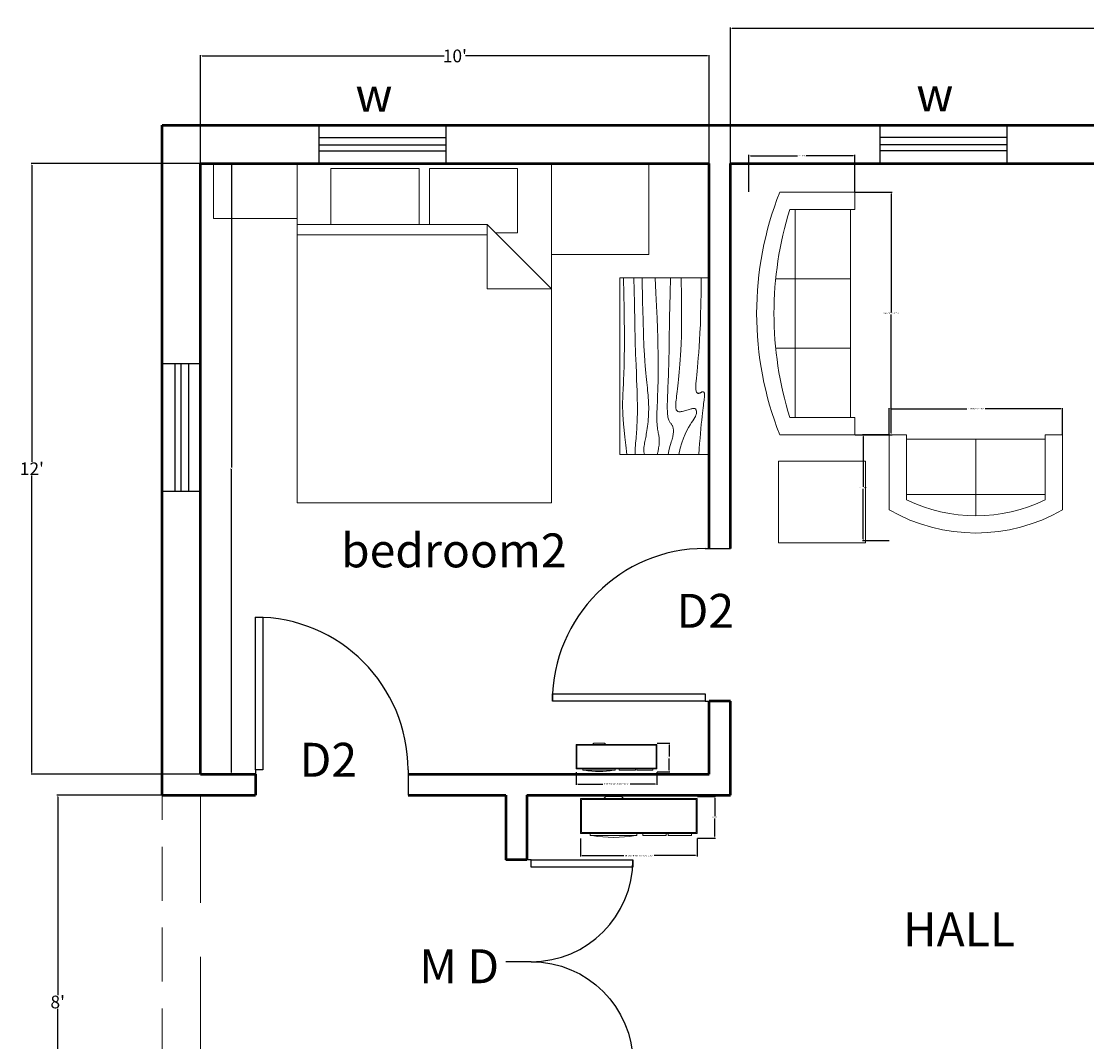
# Model space of a CAD drawing. Units: inches. Extents: x -10 to 557, y -66 to 886.
# Tile 2 of 6: x -10 to 241, y 207 to 448. Entities that reach past the tile are written whole.
import ezdxf

# ---------------------------------------------------------------- set-up
doc = ezdxf.new("R2010")
doc.units = ezdxf.units.IN
doc.header["$MEASUREMENT"] = 0
doc.linetypes.add('DASHED', pattern=[19.05, 12.7, -6.35])
for name, color, linetype, lineweight in [('A-ANNO-DIMS', 2, 'Continuous', 18), ('A-ANNO-TEXT', 7, 'Continuous', 18), ('A-AREA-IDEN', 7, 'Continuous', 25), ('A-DOOR', 4, 'Continuous', 25), ('A-FURN', 8, 'Continuous', 18), ('A-GLAZ', 4, 'Continuous', 25), ('A-WALL', 7, 'Continuous', 50), ('A-WALL-OVHD', 8, 'DASHED', 18)]:
    doc.layers.add(name, color=color, linetype=linetype, lineweight=lineweight)
doc.styles.get("Standard").update_dxf_attribs({"font": 'arial.ttf'})
doc.dimstyles.get("Standard").update_dxf_attribs({"dimtxt": 0.3, "dimasz": 0.4, "dimexe": 0.18, "dimexo": 0.0625, "dimgap": 0.09, "dimtad": 0, "dimtih": 1, "dimtoh": 1, "dimdec": 0, "dimrnd": 8, "dimzin": 0, "dimdsep": 46, "dimlunit": 3, "dimtxsty": 'Standard', "dimcen": 0.09, "dimadec": 0, "dimazin": 0, "dimtfac": 1, "dimtdec": 0, "dimtofl": 0, "dimtmove": 0, "dimatfit": 3, "dimfxl": 1, "dimtolj": 1, "dimtzin": 0, "dimarcsym": 0})

# ---------------------------------------------------------------- blocks, each defined once
blk = doc.blocks.new('*U32')
for p, q in [((0, 0), (0, -6)), ((36, 0), (36, -6))]:
    blk.add_line(p, q)
blk.add_lwpolyline([(0, 0), (0, 36), (1.75, 36), (1.75, 0)], close=True)
blk.add_arc((0, 0), 36, 0, 90)
blk = doc.blocks.new('*U33')
for p, q in [((0, 0), (0, -6)), ((24, 0), (24, -6))]:
    blk.add_line(p, q)
blk.add_lwpolyline([(0, 0), (0, 24), (1.75, 24), (1.75, 0)], close=True)
blk.add_arc((0, 0), 24, 0, 90)
blk = doc.blocks.new('Bed - Queen')
for p, q in [((0, -80.00003), (0, 0)), ((0, 0), (59.99999, 0)), ((59.99999, 0), (59.99999, -80.00003)), ((7.99999, -1.2), (28.79998, -1.2)), ((7.99999, -14.4), (7.99999, -1.2)), ((28.79998, -1.2), (28.79998, -14.4)), ((31.19999, -1.2), (51.99999, -1.2)), ((31.19999, -14.4), (31.19999, -1.2)), ((51.99999, -1.2), (51.99999, -16.4)), ((0, -14.4), (44.8, -14.4)), ((59.99999, -29.6), (44.8, -14.4)), ((44.8, -14.4), (44.8, -29.6)), ((44.8, -16.8), (0, -16.8)), ((51.99999, -16.4), (46.79936, -16.4)), ((44.8, -29.6), (59.99999, -29.6)), ((59.99999, -80.00003), (0, -80.00003))]:
    blk.add_line(p, q)
blk = doc.blocks.new('Table - Rectangular Woodgrain 60 x 30 in.')
for p, q in [((0, 0), (0, -30)), ((60, 0), (0, 0)), ((60, -30), (60, 0)), ((0, -30), (60, -30))]:
    blk.add_line(p, q)
for points in [[(0, -2.4), (4.8155, -2.418), (9.0302, -2.4688), (12.709, -2.5477), (15.9167, -2.65), (18.7181, -2.7711), (21.1781, -2.9063), (23.3616, -3.0508), (25.3333, -3.2), (27.1477, -3.3495), (28.8172, -3.4958), (30.3437, -3.636), (31.7291, -3.7667), (32.9756, -3.8849), (34.0849, -3.9875), (35.059, -4.0714), (35.9, -4.1334), (36.6114, -4.1711), (37.2041, -4.1854), (37.6906, -4.1779), (38.0833, -4.15), (38.3948, -4.1034), (38.6375, -4.0396), (38.8239, -3.9602), (38.9666, -3.8667), (39.0764, -3.7608), (39.1573, -3.6448), (39.2116, -3.521), (39.2416, -3.3917), (39.2498, -3.2593), (39.2385, -3.1261), (39.21, -2.9944), (39.1666, -2.8667), (39.111, -2.7447), (39.0468, -2.6281), (38.978, -2.5163), (38.9083, -2.4083), (38.8418, -2.3035), (38.7823, -2.201), (38.7337, -2.1001), (38.7, -2), (38.6844, -1.9003), (38.6875, -1.8021), (38.7094, -1.707), (38.75, -1.6167), (38.8094, -1.5326), (38.8875, -1.4563), (38.9844, -1.3893), (39.1, -1.3333), (39.2351, -1.2896), (39.3937, -1.2583), (39.5804, -1.2396), (39.8, -1.2333), (40.057, -1.2396), (40.3562, -1.2583), (40.7023, -1.2896), (41.1, -1.3333), (41.5547, -1.3895), (42.0755, -1.4573), (42.6721, -1.5361), (43.3542, -1.625), (44.1316, -1.7233), (45.014, -1.8302), (46.0114, -1.9449), (47.1333, -2.0667), (48.3862, -2.1947), (49.7625, -2.3281), (51.2513, -2.4663), (52.8416, -2.6083), (54.5226, -2.7535), (56.2833, -2.9011), (58.1127, -3.0501), (60, -3.2)], [(0, -9.2), (6.5759, -9.0858), (11.9385, -9.0365), (16.2527, -9.0418), (19.6833, -9.0917), (22.3952, -9.1759), (24.5531, -9.2844), (26.322, -9.4069), (27.8666, -9.5333), (29.3241, -9.6553), (30.7203, -9.7719), (32.0532, -9.8837), (33.3208, -9.9917), (34.5213, -10.0965), (35.6526, -10.199), (36.7128, -10.2999), (37.7, -10.4), (38.6129, -10.4996), (39.4531, -10.5969), (40.223, -10.6895), (40.925, -10.775), (41.5613, -10.8512), (42.1344, -10.9156), (42.6465, -10.966), (43.1, -11), (43.4976, -11.0158), (43.8437, -11.0136), (44.143, -10.9942), (44.4, -10.9583), (44.6195, -10.9069), (44.8062, -10.8406), (44.9648, -10.7603), (45.1, -10.6667), (45.2155, -10.5598), (45.3114, -10.4365), (45.3871, -10.2929), (45.4416, -10.125), (45.4743, -9.929), (45.4844, -9.7011), (45.4709, -9.4371), (45.4333, -9.1333), (45.3716, -8.7883), (45.2896, -8.4104), (45.1919, -8.0107), (45.0833, -7.6), (44.9685, -7.1893), (44.8521, -6.7896), (44.7388, -6.4117), (44.6333, -6.0667), (44.54, -5.7628), (44.4614, -5.4979), (44.4001, -5.2675), (44.3583, -5.0667), (44.3384, -4.8909), (44.3427, -4.7354), (44.3736, -4.5956), (44.4333, -4.4667), (44.5236, -4.3453), (44.6427, -4.2333), (44.7884, -4.1339), (44.9583, -4.05), (45.1501, -3.9849), (45.3614, -3.9417), (45.59, -3.9234), (45.8333, -3.9333), (46.0915, -3.9749), (46.3734, -4.0531), (46.6906, -4.1736), (47.0542, -4.3417), (47.4756, -4.5629), (47.9661, -4.8427), (48.5372, -5.1866), (49.2, -5.6), (49.9676, -6.0844), (50.8594, -6.625), (51.8965, -7.2031), (53.1, -7.8), (54.491, -8.3969), (56.0906, -8.975), (57.9199, -9.5156), (60, -10)], [(0, -12.8), (5.1847, -12.9322), (9.6213, -13.0323), (13.3963, -13.1059), (16.5958, -13.1583), (19.3063, -13.1952), (21.614, -13.2219), (23.6054, -13.2439), (25.3666, -13.2667), (26.9728, -13.2947), (28.4531, -13.3281), (29.8256, -13.3663), (31.1083, -13.4083), (32.3191, -13.4535), (33.476, -13.501), (34.597, -13.5501), (35.7, -13.6), (36.7984, -13.6497), (37.8875, -13.6979), (38.9578, -13.743), (40, -13.7833), (41.0047, -13.8174), (41.9625, -13.8438), (42.864, -13.8607), (43.7, -13.8667), (44.4631, -13.8604), (45.1552, -13.8417), (45.7801, -13.8104), (46.3416, -13.7667), (46.8439, -13.7104), (47.2906, -13.6417), (47.6858, -13.5604), (48.0333, -13.4667), (48.3375, -13.3608), (48.6042, -13.2448), (48.8396, -13.121), (49.05, -12.9917), (49.2417, -12.8593), (49.4208, -12.7261), (49.5937, -12.5944), (49.7667, -12.4667), (49.9452, -12.3451), (50.1323, -12.2313), (50.3303, -12.1268), (50.5416, -12.0333), (50.7686, -11.9524), (51.0135, -11.8854), (51.2788, -11.8341), (51.5666, -11.8), (51.8785, -11.7843), (52.2116, -11.7865), (52.562, -11.8059), (52.926, -11.8417), (53.2998, -11.8931), (53.6795, -11.9594), (54.0614, -12.0397), (54.4416, -12.1333), (54.8223, -12.2401), (55.2293, -12.3625), (55.6942, -12.5037), (56.2489, -12.6667), (56.9251, -12.8547), (57.7545, -13.0708), (58.7689, -13.3182), (60, -13.6)], [(0, -18), (5.124, -17.7273), (9.6609, -17.5057), (13.6705, -17.3303), (17.2125, -17.1958), (20.3467, -17.0973), (23.1328, -17.0297), (25.6307, -16.9878), (27.9, -16.9667), (29.9928, -16.9617), (31.9302, -16.9703), (33.7254, -16.9907), (35.3917, -17.0208), (36.9423, -17.0588), (38.3906, -17.1026), (39.7499, -17.1503), (41.0333, -17.2), (42.2519, -17.2496), (43.4073, -17.2969), (44.4986, -17.3395), (45.525, -17.375), (46.4858, -17.4012), (47.3802, -17.4156), (48.2074, -17.416), (48.9667, -17.4), (49.6583, -17.3662), (50.2872, -17.3167), (50.8595, -17.2547), (51.3812, -17.1833), (51.8584, -17.1057), (52.2971, -17.025), (52.7034, -16.9443), (53.0833, -16.8667), (53.443, -16.7951), (53.789, -16.7313), (54.128, -16.6768), (54.4666, -16.6334), (54.8115, -16.6024), (55.1693, -16.5854), (55.5465, -16.5841), (55.95, -16.6), (56.3828, -16.6337), (56.8346, -16.6823), (57.2915, -16.7418), (57.7396, -16.8084), (58.165, -16.878), (58.5539, -16.9469), (58.8924, -17.0111), (59.1666, -17.0667), (59.3679, -17.1107), (59.5078, -17.1438), (59.6032, -17.1675), (59.6708, -17.1833), (59.7275, -17.193), (59.7901, -17.1979), (59.8753, -17.1998), (60, -17.2)], [(0, -22.4), (8.0098, -22.2501), (14.4094, -22.1011), (19.4168, -21.9535), (23.25, -21.8083), (26.1269, -21.6663), (28.2656, -21.5281), (29.884, -21.3947), (31.2, -21.2667), (32.3967, -21.1448), (33.5172, -21.0292), (34.5697, -20.9198), (35.5625, -20.8167), (36.5037, -20.7198), (37.4015, -20.6292), (38.2642, -20.5448), (39.1, -20.4667), (39.9164, -20.3951), (40.7187, -20.3313), (41.5117, -20.2768), (42.3, -20.2333), (43.0883, -20.2024), (43.8812, -20.1854), (44.6836, -20.1841), (45.5, -20.2), (46.3328, -20.234), (47.1747, -20.2844), (48.0163, -20.3488), (48.8479, -20.425), (49.66, -20.5106), (50.4429, -20.6031), (51.1872, -20.7004), (51.8833, -20.8), (52.5246, -20.8999), (53.1166, -20.9995), (53.6681, -21.0983), (54.1875, -21.1958), (54.6834, -21.2919), (55.1646, -21.3859), (55.6394, -21.4777), (56.1167, -21.5667), (56.6028, -21.6515), (57.0961, -21.7266), (57.5929, -21.7852), (58.0896, -21.8208), (58.5823, -21.8268), (59.0674, -21.7964), (59.5412, -21.723), (60, -21.6)], [(0, -25.2), (8.6355, -25.0504), (15.7026, -24.9031), (21.4049, -24.7606), (25.9458, -24.625), (29.529, -24.4988), (32.3578, -24.3844), (34.6359, -24.284), (36.5667, -24.2), (38.3213, -24.1341), (39.9417, -24.0854), (41.437, -24.0523), (42.8167, -24.0333), (44.0901, -24.0268), (45.2667, -24.0313), (46.3557, -24.0451), (47.3667, -24.0667), (48.309, -24.0947), (49.1928, -24.1287), (50.0284, -24.168), (50.826, -24.2125), (51.5959, -24.2617), (52.3483, -24.3151), (53.0935, -24.3725), (53.8417, -24.4334), (54.6009, -24.497), (55.3699, -24.561), (56.1454, -24.6226), (56.9239, -24.6792), (57.7021, -24.7279), (58.4764, -24.7662), (59.2435, -24.7911), (60, -24.8)], [(0, -28.8), (5.6867, -28.6681), (10.45, -28.5698), (14.407, -28.5012), (17.675, -28.4584), (20.3711, -28.4374), (22.6125, -28.4344), (24.5164, -28.4455), (26.2, -28.4667), (27.762, -28.4947), (29.2276, -28.5281), (30.6033, -28.5663), (31.8958, -28.6084), (33.1118, -28.6535), (34.2578, -28.7011), (35.3405, -28.7501), (36.3666, -28.8), (37.3443, -28.8497), (38.288, -28.8974), (39.2137, -28.9412), (40.1375, -28.9792), (41.0753, -29.0093), (42.0432, -29.0297), (43.0572, -29.0384), (44.1333, -29.0333), (45.2936, -29.0114), (46.5843, -28.9641), (48.0579, -28.8816), (49.7666, -28.7542), (51.7629, -28.5721), (54.0989, -28.3255), (56.8272, -28.0048), (60, -27.6)]]:
    blk.add_lwpolyline(points)
blk = doc.blocks.new('Sofa - Roundback 7 ft.')
for p, q in [((-12.00002, -32.4421), (-12.00003, -6.5971)), ((11.99997, -32.4421), (11.99998, -6.5971)), ((-36.000027, -34), (-36.000027, -11.4696)), ((-35.999844, -13.3819), (35.9998, -13.3819)), ((35.99998, -34), (35.99998, -11.4696)), ((-36.000027, -32.4421), (35.99998, -32.4421))]:
    blk.add_line(p, q)
for points in [[(-36.000027, -34), (-42.000027, -34), (-42.000027, -8)], [(41.99998, -8), (41.99998, -34), (35.99998, -34)]]:
    blk.add_lwpolyline(points)
for centre, radius, start, end in [((0, -114.25), 114.25, 68.43141, 111.5686), ((-0.00001, -127.1968), 121.1968, 72.72033, 107.2797)]:
    blk.add_arc(centre, radius, start, end)
blk = doc.blocks.new('Sofa - Roundback Loveseat 5 ft.')
for p, q in [((0, -32.44198), (0, -5.99998)), ((-24, -33.99998), (-24, -11.46958)), ((-23.9998, -13.38178), (23.99986, -13.38178)), ((24.00004, -33.99998), (24.00004, -11.46958)), ((-24, -32.44198), (24.00004, -32.44198))]:
    blk.add_line(p, q)
for points in [[(-24, -33.99998), (-30, -33.99998), (-30, -7.99998)], [(30.00004, -7.99998), (30.00004, -33.99998), (24.00004, -33.99998)]]:
    blk.add_lwpolyline(points)
for centre, radius, start, end in [((0, -60.24998), 60.24998, 60.13715, 119.8628), ((0, -61.38438), 55.38444, 64.32083, 115.6792)]:
    blk.add_arc(centre, radius, start, end)
blk = doc.blocks.new('*D37')
at = {"layer": 'A-ANNO-DIMS', "color": 0, "lineweight": -2, "ltscale": 2, "transparency": 16777216}
for p, q in [((43.09, 414.4), (39.13, 414.4)), ((39.31, 414), (39.31, 342.6)), ((39.31, 270.72), (39.31, 342.12)), ((38.51, 270.32), (39.49, 270.32))]:
    blk.add_line(p, q, dxfattribs=at)
at = {"layer": 'A-ANNO-DIMS', "color": 0, "ltscale": 2, "transparency": 16777216}
for points in [[(39.25, 414), (39.38, 414), (39.31, 414.4)], [(39.25, 270.72), (39.38, 270.72), (39.31, 270.32)]]:
    blk.add_solid(points, dxfattribs=at)
at = {"layer": 'Defpoints', "color": 0, "ltscale": 2, "transparency": 16777216}
for p in [(43.15, 414.4), (38.45, 270.32), (39.31, 270.32)]:
    blk.add_point(p, dxfattribs=at)
at = {"layer": 'A-ANNO-DIMS', "color": 0, "ltscale": 2, "transparency": 16777216, "insert": (39.31, 342.36), "char_height": 0.3, "attachment_point": 5}
blk.add_mtext("\\A1;12'", dxfattribs=at)
blk = doc.blocks.new('*D38')
at = {"layer": 'A-ANNO-DIMS', "color": 0, "lineweight": -2, "ltscale": 2, "transparency": 16777216}
for p, q in [((50.7, 414.32), (-7.96, 414.32)), ((-7.78, 413.92), (-7.78, 343.92)), ((-7.78, 270.72), (-7.78, 340.73)), ((43.17, 270.32), (-7.96, 270.32))]:
    blk.add_line(p, q, dxfattribs=at)
at = {"layer": 'A-ANNO-DIMS', "color": 0, "ltscale": 2, "transparency": 16777216}
for points in [[(-7.85, 413.92), (-7.72, 413.92), (-7.78, 414.32)], [(-7.85, 270.72), (-7.72, 270.72), (-7.78, 270.32)]]:
    blk.add_solid(points, dxfattribs=at)
at = {"layer": 'Defpoints', "color": 0, "ltscale": 2, "transparency": 16777216}
for p in [(50.76, 414.32), (-7.78, 270.32), (43.23, 270.32)]:
    blk.add_point(p, dxfattribs=at)
at = {"layer": 'A-ANNO-DIMS', "color": 0, "ltscale": 2, "transparency": 16777216, "insert": (-7.78, 342.32), "char_height": 0.3, "attachment_point": 5}
blk.add_mtext("\\A1;{\\H10x;12'}", dxfattribs=at)
blk = doc.blocks.new('*D39')
at = {"layer": 'A-ANNO-DIMS', "color": 0, "lineweight": -2, "ltscale": 2, "transparency": 16777216}
for p, q in [((31.97, 414.38), (31.97, 439.85)), ((32.37, 439.67), (89.47, 439.67)), ((151.57, 439.67), (94.46, 439.67)), ((151.97, 414.38), (151.97, 439.85))]:
    blk.add_line(p, q, dxfattribs=at)
at = {"layer": 'A-ANNO-DIMS', "color": 0, "ltscale": 2, "transparency": 16777216}
for points in [[(32.37, 439.74), (32.37, 439.61), (31.97, 439.67)], [(151.57, 439.74), (151.57, 439.61), (151.97, 439.67)]]:
    blk.add_solid(points, dxfattribs=at)
at = {"layer": 'Defpoints', "color": 0, "ltscale": 2, "transparency": 16777216}
for p in [(151.97, 439.67), (31.97, 414.32), (151.97, 414.32)]:
    blk.add_point(p, dxfattribs=at)
at = {"layer": 'A-ANNO-DIMS', "color": 0, "ltscale": 2, "transparency": 16777216, "insert": (91.97, 439.67), "char_height": 0.3, "attachment_point": 5}
blk.add_mtext("\\A1;{\\H10x;10'}", dxfattribs=at)
blk = doc.blocks.new('*D40')
at = {"layer": 'A-ANNO-DIMS', "color": 0, "lineweight": -2, "ltscale": 2, "transparency": 16777216}
for p, q in [((156.97, 414.38), (156.97, 446.36)), ((157.37, 446.18), (298.2, 446.18)), ((449.57, 446.18), (308.74, 446.18)), ((449.97, 414.38), (449.97, 446.36))]:
    blk.add_line(p, q, dxfattribs=at)
at = {"layer": 'A-ANNO-DIMS', "color": 0, "ltscale": 2, "transparency": 16777216}
for points in [[(157.37, 446.25), (157.37, 446.11), (156.97, 446.18)], [(449.57, 446.25), (449.57, 446.11), (449.97, 446.18)]]:
    blk.add_solid(points, dxfattribs=at)
at = {"layer": 'Defpoints', "color": 0, "ltscale": 2, "transparency": 16777216}
for p in [(449.97, 446.18), (156.97, 414.32), (449.97, 414.32)]:
    blk.add_point(p, dxfattribs=at)
at = {"layer": 'A-ANNO-DIMS', "color": 0, "ltscale": 2, "transparency": 16777216, "insert": (303.47, 446.18), "char_height": 0.3, "attachment_point": 5}
blk.add_mtext('\\A1;{\\H10x;24\'-8"}', dxfattribs=at)
blk = doc.blocks.new('*D42')
at = {"layer": 'A-ANNO-DIMS', "color": 0, "lineweight": -2, "ltscale": 2, "transparency": 16777216}
for p, q in [((31.91, 265.32), (-1.86, 265.32)), ((-1.68, 264.92), (-1.68, 218.2)), ((-1.68, 168.23), (-1.68, 214.95)), ((31.91, 167.83), (-1.86, 167.83))]:
    blk.add_line(p, q, dxfattribs=at)
at = {"layer": 'A-ANNO-DIMS', "color": 0, "ltscale": 2, "transparency": 16777216}
for points in [[(-1.75, 264.92), (-1.61, 264.92), (-1.68, 265.32)], [(-1.75, 168.23), (-1.61, 168.23), (-1.68, 167.83)]]:
    blk.add_solid(points, dxfattribs=at)
at = {"layer": 'Defpoints', "color": 0, "ltscale": 2, "transparency": 16777216}
for p in [(31.97, 265.32), (-1.68, 167.83), (31.97, 167.83)]:
    blk.add_point(p, dxfattribs=at)
at = {"layer": 'A-ANNO-DIMS', "color": 0, "ltscale": 2, "transparency": 16777216, "insert": (-1.68, 216.57), "char_height": 0.3, "attachment_point": 5}
blk.add_mtext("\\A1;{\\H10x;8'}", dxfattribs=at)
blk = doc.blocks.new('Entertainment Center')
for p, q in [((-4, 0), (-5, -1)), ((4, 0), (-4, 0)), ((5, -1), (4, 0)), ((-17, -19), (-17, -1)), ((-17, -1), (43, -1)), ((-16.5, -18.5), (-16.5, -1.5)), ((-16.5, -1.5), (42.5, -1.5)), ((42.5, -1.5), (42.5, -18.5)), ((43, -1), (43, -19)), ((43, -19), (-17, -19)), ((42.5, -18.5), (-16.5, -18.5)), ((-12, -20), (-12, -19)), ((12, -20), (-12, -20)), ((12, -19), (12, -20)), ((15, -20), (15, -19)), ((27, -20), (15, -20)), ((27, -19), (27, -20)), ((28, -20), (28, -19)), ((40, -20), (28, -20)), ((40, -19), (40, -20))]:
    blk.add_line(p, q)
blk.add_arc((0, 40), 61, 259.6111, 280.3889)
blk = doc.blocks.new('WIN-900')
for p, q in [((0, 6.25), (30, 6.25)), ((0, 4.5), (30, 4.5)), ((0, 3.05), (30, 3.05))]:
    blk.add_line(p, q)
blk.add_lwpolyline([(0, 9), (0, 0), (30, 0), (30, 9)], close=True)
blk = doc.blocks.new('*D61')
at = {"layer": 'A-ANNO-DIMS', "color": 0, "lineweight": -2, "ltscale": 2, "transparency": 16777216}
for p, q in [((121.62, 255.16), (121.62, 250.92)), ((149.13, 255.16), (149.13, 250.92)), ((122.02, 251.1), (131.79, 251.1)), ((148.73, 251.1), (138.97, 251.1))]:
    blk.add_line(p, q, dxfattribs=at)
at = {"layer": 'A-ANNO-DIMS', "color": 0, "ltscale": 2, "transparency": 16777216}
for points in [[(122.02, 251.16), (122.02, 251.03), (121.62, 251.1)], [(148.73, 251.16), (148.73, 251.03), (149.13, 251.1)]]:
    blk.add_solid(points, dxfattribs=at)
at = {"layer": 'Defpoints', "color": 0, "ltscale": 2, "transparency": 16777216}
for p in [(121.62, 255.22), (149.13, 255.22), (149.13, 251.1)]:
    blk.add_point(p, dxfattribs=at)
at = {"layer": 'A-ANNO-DIMS', "color": 0, "ltscale": 2, "transparency": 16777216, "insert": (135.38, 251.1), "char_height": 0.3, "attachment_point": 5}
blk.add_mtext('\\A1;ENTERTAINMENT CENTER 2\'-3 1/2"', dxfattribs=at)
blk = doc.blocks.new('*D62')
at = {"layer": 'A-ANNO-DIMS', "color": 0, "lineweight": -2, "ltscale": 2, "transparency": 16777216}
for p, q in [((149.2, 265.01), (153.44, 265.01)), ((153.26, 264.61), (153.26, 260.36)), ((153.26, 255.62), (153.26, 259.87)), ((149.2, 255.22), (153.44, 255.22))]:
    blk.add_line(p, q, dxfattribs=at)
at = {"layer": 'A-ANNO-DIMS', "color": 0, "ltscale": 2, "transparency": 16777216}
for points in [[(153.19, 264.61), (153.33, 264.61), (153.26, 265.01)], [(153.19, 255.62), (153.33, 255.62), (153.26, 255.22)]]:
    blk.add_solid(points, dxfattribs=at)
at = {"layer": 'Defpoints', "color": 0, "ltscale": 2, "transparency": 16777216}
for p in [(149.13, 265.01), (153.26, 265.01), (149.13, 255.22)]:
    blk.add_point(p, dxfattribs=at)
at = {"layer": 'A-ANNO-DIMS', "color": 0, "ltscale": 2, "transparency": 16777216, "insert": (153.26, 260.11), "char_height": 0.3, "attachment_point": 5}
blk.add_mtext('\\A1;0\'-10"', dxfattribs=at)
blk = doc.blocks.new('*D63')
at = {"layer": 'A-ANNO-DIMS', "color": 0, "lineweight": -2, "ltscale": 2, "transparency": 16777216}
for p, q in [((120.6, 270.77), (120.6, 267.8)), ((139.63, 270.77), (139.63, 267.8)), ((121, 267.98), (126.87, 267.98)), ((139.23, 267.98), (133.35, 267.98))]:
    blk.add_line(p, q, dxfattribs=at)
at = {"layer": 'A-ANNO-DIMS', "color": 0, "ltscale": 2, "transparency": 16777216}
for points in [[(121, 268.04), (121, 267.91), (120.6, 267.98)], [(139.23, 268.04), (139.23, 267.91), (139.63, 267.98)]]:
    blk.add_solid(points, dxfattribs=at)
at = {"layer": 'Defpoints', "color": 0, "ltscale": 2, "transparency": 16777216}
for p in [(120.6, 270.83), (139.63, 270.83), (139.63, 267.98)]:
    blk.add_point(p, dxfattribs=at)
at = {"layer": 'A-ANNO-DIMS', "color": 0, "ltscale": 2, "transparency": 16777216, "insert": (130.11, 267.98), "char_height": 0.3, "attachment_point": 5}
blk.add_mtext('\\A1;ENTERTAINMENT CENTER 1\'-7"', dxfattribs=at)
blk = doc.blocks.new('*D64')
at = {"layer": 'A-ANNO-DIMS', "color": 0, "lineweight": -2, "ltscale": 2, "transparency": 16777216}
for p, q in [((139.69, 277.6), (142.67, 277.6)), ((142.49, 277.2), (142.49, 274.46)), ((142.49, 271.23), (142.49, 273.97)), ((139.69, 270.83), (142.67, 270.83))]:
    blk.add_line(p, q, dxfattribs=at)
at = {"layer": 'A-ANNO-DIMS', "color": 0, "ltscale": 2, "transparency": 16777216}
for points in [[(142.42, 277.2), (142.55, 277.2), (142.49, 277.6)], [(142.42, 271.23), (142.55, 271.23), (142.49, 270.83)]]:
    blk.add_solid(points, dxfattribs=at)
at = {"layer": 'Defpoints', "color": 0, "ltscale": 2, "transparency": 16777216}
for p in [(139.63, 277.6), (142.49, 277.6), (139.63, 270.83)]:
    blk.add_point(p, dxfattribs=at)
at = {"layer": 'A-ANNO-DIMS', "color": 0, "ltscale": 2, "transparency": 16777216, "insert": (142.49, 274.21), "char_height": 0.3, "attachment_point": 5}
blk.add_mtext('\\A1;0\'-7"', dxfattribs=at)
blk = doc.blocks.new('*D71')
at = {"layer": 'A-ANNO-DIMS', "color": 0, "lineweight": -2, "ltscale": 2, "transparency": 16777216}
for p, q in [((186.36, 407.56), (195.07, 407.56)), ((194.89, 407.16), (194.89, 379.19)), ((194.89, 350.73), (194.89, 378.7)), ((186.36, 350.33), (195.07, 350.33))]:
    blk.add_line(p, q, dxfattribs=at)
at = {"layer": 'A-ANNO-DIMS', "color": 0, "ltscale": 2, "transparency": 16777216}
for points in [[(194.82, 407.16), (194.95, 407.16), (194.89, 407.56)], [(194.82, 350.73), (194.95, 350.73), (194.89, 350.33)]]:
    blk.add_solid(points, dxfattribs=at)
at = {"layer": 'Defpoints', "color": 0, "ltscale": 2, "transparency": 16777216}
for p in [(186.3, 407.56), (194.89, 407.56), (186.3, 350.33)]:
    blk.add_point(p, dxfattribs=at)
at = {"layer": 'A-ANNO-DIMS', "color": 0, "ltscale": 2, "transparency": 16777216, "insert": (194.89, 378.94), "char_height": 0.3, "attachment_point": 5}
blk.add_mtext('\\A1;SOFA 7 FT 4\'-9" TYP.', dxfattribs=at)
blk = doc.blocks.new('*D72')
at = {"layer": 'A-ANNO-DIMS', "color": 0, "lineweight": -2, "ltscale": 2, "transparency": 16777216}
for p, q in [((161.32, 407.62), (161.32, 416.32)), ((161.72, 416.14), (172.8, 416.14)), ((185.9, 416.14), (174.82, 416.14)), ((186.3, 407.62), (186.3, 416.32))]:
    blk.add_line(p, q, dxfattribs=at)
at = {"layer": 'A-ANNO-DIMS', "color": 0, "ltscale": 2, "transparency": 16777216}
for points in [[(161.72, 416.21), (161.72, 416.08), (161.32, 416.14)], [(185.9, 416.21), (185.9, 416.08), (186.3, 416.14)]]:
    blk.add_solid(points, dxfattribs=at)
at = {"layer": 'Defpoints', "color": 0, "ltscale": 2, "transparency": 16777216}
for p in [(161.32, 416.14), (161.32, 407.56), (186.3, 407.56)]:
    blk.add_point(p, dxfattribs=at)
at = {"layer": 'A-ANNO-DIMS', "color": 0, "ltscale": 2, "transparency": 16777216, "insert": (173.81, 416.14), "char_height": 0.3, "attachment_point": 5}
blk.add_mtext('\\A1;2\'-1" TYP.', dxfattribs=at)
blk = doc.blocks.new('*D73')
at = {"layer": 'A-ANNO-DIMS', "color": 0, "lineweight": -2, "ltscale": 2, "transparency": 16777216}
for p, q in [((194.42, 350.39), (194.42, 356.64)), ((194.82, 356.46), (212.7, 356.46)), ((234.9, 356.46), (217.02, 356.46)), ((235.3, 350.39), (235.3, 356.64))]:
    blk.add_line(p, q, dxfattribs=at)
at = {"layer": 'A-ANNO-DIMS', "color": 0, "ltscale": 2, "transparency": 16777216}
for points in [[(194.82, 356.53), (194.82, 356.4), (194.42, 356.46)], [(234.9, 356.53), (234.9, 356.4), (235.3, 356.46)]]:
    blk.add_solid(points, dxfattribs=at)
at = {"layer": 'Defpoints', "color": 0, "ltscale": 2, "transparency": 16777216}
for p in [(194.42, 356.46), (194.42, 350.33), (235.3, 350.33)]:
    blk.add_point(p, dxfattribs=at)
at = {"layer": 'A-ANNO-DIMS', "color": 0, "ltscale": 2, "transparency": 16777216, "insert": (214.86, 356.46), "char_height": 0.3, "attachment_point": 5}
blk.add_mtext('\\A1;LOVESEAT 3\'-5" TYP.', dxfattribs=at)
blk = doc.blocks.new('*D74')
at = {"layer": 'A-ANNO-DIMS', "color": 0, "lineweight": -2, "ltscale": 2, "transparency": 16777216}
for p, q in [((194.36, 350.33), (188.11, 350.33)), ((188.29, 349.93), (188.29, 338.08)), ((188.29, 325.75), (188.29, 337.6)), ((194.36, 325.35), (188.11, 325.35))]:
    blk.add_line(p, q, dxfattribs=at)
at = {"layer": 'A-ANNO-DIMS', "color": 0, "ltscale": 2, "transparency": 16777216}
for points in [[(188.22, 349.93), (188.36, 349.93), (188.29, 350.33)], [(188.22, 325.75), (188.36, 325.75), (188.29, 325.35)]]:
    blk.add_solid(points, dxfattribs=at)
at = {"layer": 'Defpoints', "color": 0, "ltscale": 2, "transparency": 16777216}
for p in [(194.42, 350.33), (188.29, 325.35), (194.42, 325.35)]:
    blk.add_point(p, dxfattribs=at)
at = {"layer": 'A-ANNO-DIMS', "color": 0, "ltscale": 2, "transparency": 16777216, "insert": (188.29, 337.84), "char_height": 0.3, "attachment_point": 5}
blk.add_mtext('\\A1;2\'-1" TYP.', dxfattribs=at)

msp = doc.modelspace()

# ---------------------------------------------------------------- linework, layer by layer
at = {"layer": 'A-FURN'}
for points in [[(54.76, 414.32), (54.76, 401.3), (35.05, 401.3), (35.05, 414.32)], [(114.76, 414.32), (114.76, 392.81), (137.71, 392.81), (137.71, 414.32)], [(168.29, 344.12), (188.84, 344.12), (188.84, 324.87), (168.29, 324.87)]]:
    msp.add_lwpolyline(points, close=True, dxfattribs=at)
at = {"layer": 'A-WALL'}
for p, q in [((22.97, 423.32), (382.97, 423.32)), ((22.97, 265.28), (22.97, 423.32)), ((31.97, 414.32), (151.97, 414.32)), ((31.97, 270.32), (31.97, 414.32)), ((151.97, 323.51), (151.97, 414.32)), ((156.97, 414.32), (449.97, 414.32)), ((156.97, 323.51), (156.97, 414.32)), ((151.97, 270.32), (151.97, 287.51)), ((156.97, 287.51), (151.97, 287.51)), ((156.97, 265.32), (156.97, 287.51)), ((31.97, 270.32), (44.93, 270.32)), ((44.93, 270.32), (44.93, 265.32)), ((80.93, 270.32), (151.97, 270.32)), ((22.97, 265.32), (44.93, 265.32)), ((31.97, 265.32), (44.93, 265.32)), ((80.93, 265.32), (103.97, 265.32)), ((80.93, 265.32), (103.97, 265.32)), ((103.97, 265.32), (103.97, 250.08)), ((108.97, 265.32), (108.97, 250.08)), ((108.97, 265.32), (156.97, 265.32)), ((108.97, 250.08), (103.97, 250.08))]:
    msp.add_line(p, q, dxfattribs=at)
at = {"layer": 'A-WALL-OVHD'}
msp.add_line((22.97, 164.26), (22.97, 265.28), dxfattribs=at)
at = {"layer": 'A-WALL-OVHD', "ltscale": 2}
msp.add_line((31.97, 265.32), (31.97, 164.32), dxfattribs=at)

# ---------------------------------------------------------------- block references
at = {"layer": 'A-DOOR'}
for name, p, rotation in [('*U32', (150.97, 287.51), 90), ('*U33', (109.97, 250.08), 270)]:
    msp.add_blockref(name, p, dxfattribs=dict(at, rotation=rotation))
msp.add_blockref('*U32', (44.93, 271.32), dxfattribs=at)
at = {"layer": 'A-DOOR', "xscale": -1, "rotation": 270}
msp.add_blockref('*U33', (109.97, 202.08), dxfattribs=at)
at = {"layer": 'A-FURN'}
msp.add_blockref('Bed - Queen', (54.76, 414.32), dxfattribs=at)
for name, p, xscale, yscale, zscale, rotation in [('Sofa - Roundback 7 ft.', (163.14, 378.94), 0.6812959275706195, 0.6812959275706195, 0.6812959275706195, 90), ('Table - Rectangular Woodgrain 60 x 30 in.', (151.7, 387.35), 0.6942880543039835, 0.6942880543039835, 0.6942880543039835, 270), ('Table - Rectangular Woodgrain 60 x 30 in.', (151.7, 387.35), 0.6942880543039835, 0.6942880543039835, 0.6942880543039835, 270), ('Table - Rectangular Woodgrain 60 x 30 in.', (151.7, 387.35), 0.6942880543039835, 0.6942880543039835, 0.6942880543039835, 270), ('Table - Rectangular Woodgrain 60 x 30 in.', (151.7, 387.35), 0.6942880543039835, 0.6942880543039835, 0.6942880543039835, 270), ('Sofa - Roundback Loveseat 5 ft.', (214.86, 327.17), 0.6812959275706195, 0.6812959275706195, 0.6812959275706195, 180)]:
    msp.add_blockref(name, p, dxfattribs=dict(at, xscale=xscale, yscale=yscale, zscale=zscale, rotation=rotation))
for p, xscale, yscale, zscale in [((125.99, 277.6), 0.3172331173943709, 0.3172331173943709, 0.3172331173943709), ((129.42, 265.01), 0.4585252012591106, 0.4585252012591106, 0.4585252012591106)]:
    msp.add_blockref('Entertainment Center', p, dxfattribs=dict(at, xscale=xscale, yscale=yscale, zscale=zscale))
at = {"layer": 'A-GLAZ'}
for p in [(59.93, 414.21), (192.19, 414.29)]:
    msp.add_blockref('WIN-900', p, dxfattribs=at)
at = {"layer": 'A-GLAZ', "rotation": 270.0000000000003}
msp.add_blockref('WIN-900', (22.88, 367.05), dxfattribs=at)

# ---------------------------------------------------------------- texts
at = {"layer": 'A-ANNO-TEXT', "char_height": 8, "attachment_point": 1}
for s, insert in [('w', (68.52, 434.52)), ('w', (200.78, 434.6)), ('D2', (144.25, 312.81)), ('D2', (55.35, 277.69))]:
    msp.add_mtext_dynamic_manual_height_columns(s, width=13.506, gutter_width=1, heights=[0], dxfattribs=dict(at, insert=insert))
at = {"layer": 'A-ANNO-TEXT', "ltscale": 5, "insert": (83.59, 229), "char_height": 8, "attachment_point": 1}
msp.add_mtext_dynamic_manual_height_columns('M D', width=36.6815, gutter_width=1, heights=[0], dxfattribs=at)
at = {"layer": 'A-AREA-IDEN', "char_height": 8, "attachment_point": 1}
for s, width, insert in [('bedroom2', 38.1538, (65.13, 327.07)), ('HALL', 67.0443, (197.63, 237.68))]:
    msp.add_mtext_dynamic_manual_height_columns(s, width=width, gutter_width=1, heights=[0], dxfattribs=dict(at, insert=insert))

# ---------------------------------------------------------------- dimensions: what is measured, and where the dimension line sits
at = {"layer": 'A-ANNO-DIMS', "ltscale": 2}
for base, p1, p2, text, override, picture, middle in [((449.97, 446.18), (156.97, 414.32), (449.97, 414.32), '{\\H10x;<>}', {"dimclrd": 0, "dimclre": 0, "dimclrt": 0}, '*D40', (303.47, 446.18)), ((151.97, 439.67), (31.97, 414.32), (151.97, 414.32), '{\\H10x;<>}', {"dimclrd": 0, "dimclre": 0, "dimclrt": 0}, '*D39', (91.97, 439.67)), ((139.63, 267.98), (120.6, 270.83), (139.63, 270.83), 'ENTERTAINMENT CENTER <>', {"dimdec": 1, "dimrnd": 0, "dimzin": 1, "dimlunit": 4, "dimfrac": 2}, '*D63', (130.11, 267.98)), ((149.13, 251.1), (121.62, 255.22), (149.13, 255.22), 'ENTERTAINMENT CENTER <>', {"dimdec": 1, "dimrnd": 0, "dimzin": 1, "dimlunit": 4, "dimfrac": 2}, '*D61', (135.38, 251.1))]:
    dim = msp.add_linear_dim(base=base, p1=p1, p2=p2, text=text, dimstyle='Standard', override=override, dxfattribs=at)
    dim.commit()
    dim.dimension.update_dxf_attribs({"geometry": picture, "text_midpoint": middle})
for base, p1, p2, angle, text, override, picture, middle in [((161.32, 416.14), (186.3, 407.56), (161.32, 407.56), 180, '<> TYP.', {"dimdec": 1, "dimrnd": 0, "dimzin": 1, "dimlunit": 4, "dimfrac": 2}, '*D72', (173.81, 416.14)), ((-7.78, 270.32), (50.76, 414.32), (43.23, 270.32), 90, '{\\H10x;<>}', {"dimclrd": 0, "dimclre": 0, "dimclrt": 0}, '*D38', (-7.78, 342.32)), ((194.89, 407.56), (186.3, 350.33), (186.3, 407.56), 90, 'SOFA 7 FT <> TYP.', {"dimdec": 1, "dimrnd": 0, "dimzin": 1, "dimlunit": 4, "dimfrac": 2}, '*D71', (194.89, 378.94)), ((194.42, 356.46), (235.3, 350.33), (194.42, 350.33), 180, 'LOVESEAT <> TYP.', {"dimdec": 1, "dimrnd": 0, "dimzin": 1, "dimlunit": 4, "dimfrac": 2}, '*D73', (214.86, 356.46)), ((188.29, 325.35), (194.42, 350.33), (194.42, 325.35), 270, '<> TYP.', {"dimdec": 1, "dimrnd": 0, "dimzin": 1, "dimlunit": 4, "dimfrac": 2}, '*D74', (188.29, 337.84)), ((-1.68, 167.83), (31.97, 265.32), (31.97, 167.83), 90, '{\\H10x;<>}', {"dimclrd": 0, "dimclre": 0, "dimclrt": 0}, '*D42', (-1.68, 216.57))]:
    dim = msp.add_linear_dim(base=base, p1=p1, p2=p2, angle=angle, text=text, dimstyle='Standard', override=override, dxfattribs=at)
    dim.commit()
    dim.dimension.update_dxf_attribs({"geometry": picture, "text_midpoint": middle})
for base, p1, p2, override, picture, middle in [((39.31, 270.32), (43.15, 414.4), (38.45, 270.32), {"dimclrd": 0, "dimclre": 0, "dimclrt": 0}, '*D37', (39.31, 342.36)), ((142.49, 277.6), (139.63, 270.83), (139.63, 277.6), {"dimdec": 1, "dimrnd": 0, "dimzin": 1, "dimlunit": 4, "dimfrac": 2}, '*D64', (142.49, 274.21)), ((153.26, 265.01), (149.13, 255.22), (149.13, 265.01), {"dimdec": 1, "dimrnd": 0, "dimzin": 1, "dimlunit": 4, "dimfrac": 2}, '*D62', (153.26, 260.11))]:
    dim = msp.add_linear_dim(base=base, p1=p1, p2=p2, angle=90, dimstyle='Standard', override=override, dxfattribs=at)
    dim.commit()
    dim.dimension.update_dxf_attribs({"geometry": picture, "text_midpoint": middle})

doc.saveas('drawing.dxf')
